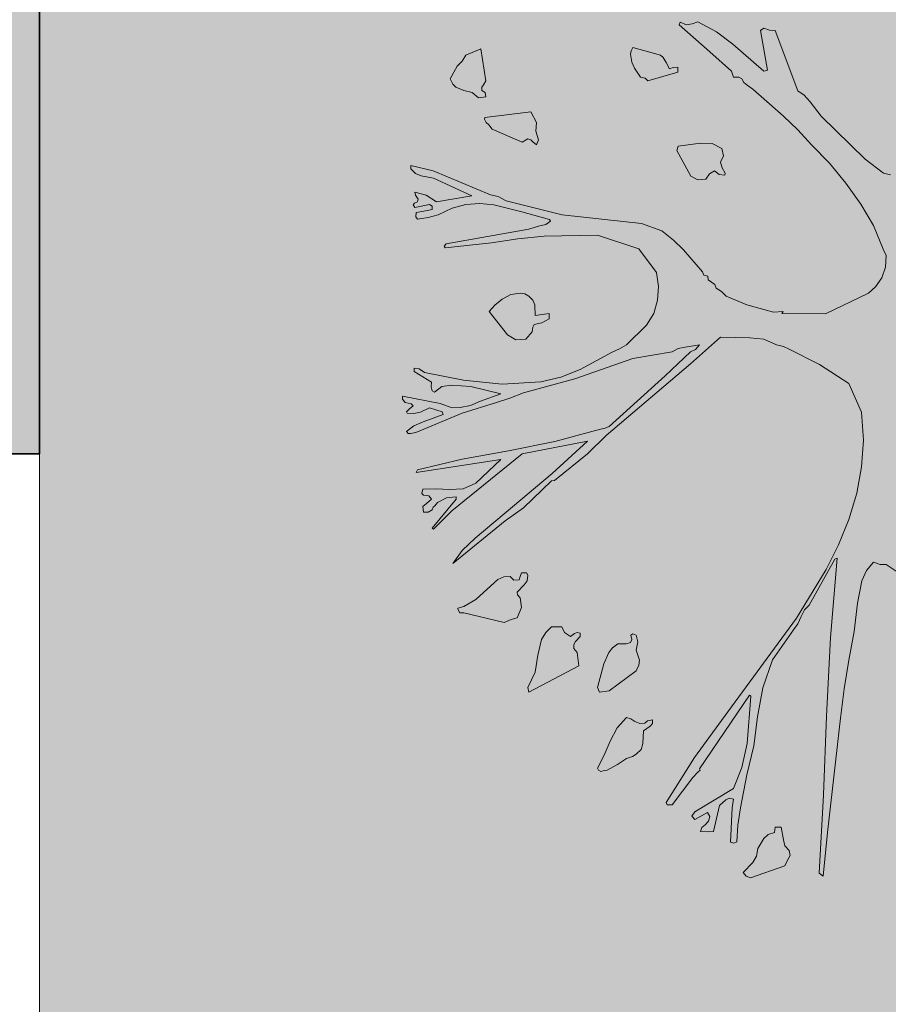
# Model space of a CAD drawing. Units: inches. Extents: x 84 to 1044, y -280 to 906.
# Tile 75 of 105: x 704 to 720, y 481 to 500. Entities that reach past the tile are written whole.
import ezdxf

# ---------------------------------------------------------------- set-up
doc = ezdxf.new("R2010")
doc.units = ezdxf.units.IN
for name, color, linetype, lineweight in [('A-ANNO-DIMS', 2, 'Continuous', 18), ('L-PLNT', 114, 'Continuous', 15), ('WALL', 250, 'Continuous', 35), ('WINDOW', 160, 'Continuous', 13)]:
    doc.layers.add(name, color=color, linetype=linetype, lineweight=lineweight)
doc.layers.add('A-WALL-PATT', color=251, linetype='Continuous', lineweight=9, true_color=0x636466)
doc.layers.add('L-PLNT-PATT', color=9, linetype='Continuous', lineweight=9, true_color=0xafd9aa)
doc.styles.get("Standard").update_dxf_attribs({"font": 'arial.ttf'})
doc.dimstyles.get("Standard").update_dxf_attribs({"dimtxt": 0.18, "dimasz": 0.18, "dimexe": 0.18, "dimexo": 0.0625, "dimgap": 0.09, "dimtad": 0, "dimtih": 1, "dimtoh": 1, "dimdec": 4, "dimzin": 0, "dimdsep": 46, "dimtxsty": 'Standard', "dimcen": 0.09, "dimadec": 0, "dimazin": 0, "dimtfac": 1, "dimtdec": 4, "dimtofl": 0, "dimtmove": 0, "dimatfit": 3, "dimfxl": 1, "dimtolj": 1, "dimtzin": 0, "dimarcsym": 0})

# ---------------------------------------------------------------- blocks, each defined once
blk = doc.blocks.new('A$C37E508DF')
for p, q in [((0.3456, 1.093), (0.3469, 1.0964)), ((0.3469, 1.0964), (0.355, 1.093)), ((0.3619, 1.0943), (0.3692, 1.0968)), ((0.3692, 1.0968), (0.3923, 1.0844)), ((0.3842, 1.0591), (0.3456, 1.093)), ((0.355, 1.093), (0.3619, 1.0943)), ((0.3923, 1.0844), (0.4129, 1.069)), ((0.4472, 1.0857), (0.4515, 1.0887)), ((0.4562, 1.0364), (0.4472, 1.0857)), ((0.4515, 1.0887), (0.4584, 1.0865)), ((0.4584, 1.0865), (0.4657, 1.0861)), ((0.4657, 1.0861), (0.4939, 1.0107)), ((0.0789, 1.0552), (0.0978, 1.063)), ((0.0978, 1.063), (0.1042, 1.0231)), ((0.2847, 1.0565), (0.2856, 1.0604)), ((0.2856, 1.0604), (0.2877, 1.0647)), ((0.2877, 1.0647), (0.3224, 1.0552)), ((0.4112, 1.0351), (0.3842, 1.0591)), ((0.4129, 1.069), (0.4515, 1.0351)), ((0.0682, 1.0415), (0.0746, 1.0475)), ((0.0746, 1.0475), (0.0789, 1.0552)), ((0.2851, 1.054), (0.2847, 1.0565)), ((0.2864, 1.0463), (0.2851, 1.054)), ((0.2899, 1.039), (0.2864, 1.0463)), ((0.3224, 1.0552), (0.3255, 1.0522)), ((0.3255, 1.0522), (0.3293, 1.0458)), ((0.3293, 1.0458), (0.3336, 1.0381)), ((0.0596, 1.0257), (0.0682, 1.0415)), ((0.2972, 1.0274), (0.2899, 1.039)), ((0.3439, 1.0338), (0.3066, 1.0231)), ((0.3336, 1.0381), (0.3383, 1.0398)), ((0.3383, 1.0398), (0.3439, 1.0402)), ((0.3439, 1.0402), (0.3439, 1.0338)), ((0.4138, 1.0274), (0.4112, 1.0351)), ((0.4515, 1.0351), (0.4562, 1.0364)), ((0.0626, 1.0188), (0.0596, 1.0257)), ((0.1042, 1.0231), (0.1012, 1.018)), ((0.3032, 1.0265), (0.2972, 1.0274)), ((0.3066, 1.0231), (0.3032, 1.0265)), ((0.4202, 1.0274), (0.4138, 1.0274)), ((0.4241, 1.0257), (0.4202, 1.0274)), ((0.4267, 1.0209), (0.4241, 1.0257)), ((0.0665, 1.0149), (0.0626, 1.0188)), ((0.0763, 1.0111), (0.0665, 1.0149)), ((0.087, 1.0085), (0.0763, 1.0111)), ((0.1012, 1.018), (0.099, 1.0149)), ((0.099, 1.0149), (0.099, 1.0111)), ((0.099, 1.0111), (0.1033, 1.0085)), ((0.4305, 1.0175), (0.4267, 1.0209)), ((0.4378, 1.0124), (0.4305, 1.0175)), ((0.476, 0.9789), (0.4378, 1.0124)), ((0.4939, 1.0107), (0.5021, 1.0051)), ((0.0948, 1.0016), (0.087, 1.0085)), ((0.1042, 1.0029), (0.0948, 1.0016)), ((0.1033, 1.0085), (0.1042, 1.0029)), ((0.5021, 1.0051), (0.5094, 0.9969)), ((0.5094, 0.9969), (0.5231, 0.9789)), ((0.1025, 0.9751), (0.1029, 0.9772)), ((0.1046, 0.9708), (0.1025, 0.9751)), ((0.1029, 0.9772), (0.1604, 0.9841)), ((0.1604, 0.9841), (0.1672, 0.9708)), ((0.4939, 0.9618), (0.476, 0.9789)), ((0.5231, 0.9789), (0.578, 0.9253)), ((0.1076, 0.9682), (0.1046, 0.9708)), ((0.1119, 0.9626), (0.1076, 0.9682)), ((0.1496, 0.9463), (0.1119, 0.9626)), ((0.1672, 0.9708), (0.1664, 0.9601)), ((0.1664, 0.9601), (0.1698, 0.9493)), ((0.5111, 0.9429), (0.4939, 0.9618)), ((0.1565, 0.9506), (0.1496, 0.9463)), ((0.1604, 0.9493), (0.1565, 0.9506)), ((0.1629, 0.9468), (0.1604, 0.9493)), ((0.1698, 0.9493), (0.1672, 0.9429)), ((0.1672, 0.9429), (0.1629, 0.9468)), ((0.3426, 0.936), (0.3443, 0.9412)), ((0.3602, 0.9039), (0.3426, 0.936)), ((0.3443, 0.9412), (0.3722, 0.9451)), ((0.3722, 0.9451), (0.3868, 0.9446)), ((0.3868, 0.9446), (0.3992, 0.9386)), ((0.3992, 0.9386), (0.4009, 0.9292)), ((0.5334, 0.9202), (0.5111, 0.9429)), ((0.4009, 0.9292), (0.3975, 0.9215)), ((0.578, 0.9253), (0.6011, 0.9077)), ((0.0103, 0.9129), (0.0103, 0.9172)), ((0.0103, 0.9172), (0.0382, 0.9107)), ((0.0159, 0.9073), (0.0103, 0.9129)), ((0.0382, 0.9107), (0.1098, 0.8807)), ((0.3898, 0.9107), (0.3838, 0.9069)), ((0.3958, 0.906), (0.3898, 0.9107)), ((0.3975, 0.9215), (0.3996, 0.9142)), ((0.3996, 0.9142), (0.4031, 0.9077)), ((0.554, 0.8953), (0.5334, 0.9202)), ((0.0232, 0.9043), (0.0159, 0.9073)), ((0.0386, 0.9013), (0.0232, 0.9043)), ((0.0866, 0.8794), (0.0386, 0.9013)), ((0.3692, 0.8992), (0.3602, 0.9039)), ((0.379, 0.9), (0.3692, 0.8992)), ((0.3838, 0.9069), (0.379, 0.9)), ((0.4026, 0.9052), (0.3958, 0.906)), ((0.4031, 0.9077), (0.4026, 0.9052)), ((0.6011, 0.9077), (0.6097, 0.9056)), ((0.5728, 0.8691), (0.554, 0.8953)), ((0.0159, 0.8803), (0.0154, 0.8837)), ((0.0154, 0.8837), (0.0292, 0.8803)), ((0.0176, 0.8777), (0.0159, 0.8803)), ((0.0193, 0.8752), (0.0176, 0.8777)), ((0.0184, 0.8717), (0.0193, 0.8752)), ((0.0292, 0.8803), (0.0424, 0.8717)), ((0.0424, 0.8717), (0.0866, 0.8794)), ((0.1098, 0.8807), (0.1196, 0.8786)), ((0.1196, 0.8786), (0.1295, 0.873)), ((0.0133, 0.8679), (0.015, 0.87)), ((0.0154, 0.8649), (0.0133, 0.8679)), ((0.015, 0.87), (0.0184, 0.8717)), ((0.0334, 0.8687), (0.0154, 0.8649)), ((0.0266, 0.8602), (0.0369, 0.8623)), ((0.0369, 0.8666), (0.0334, 0.8687)), ((0.0369, 0.8623), (0.0369, 0.8666)), ((0.0617, 0.864), (0.0442, 0.8554)), ((0.0789, 0.8687), (0.0617, 0.864)), ((0.0965, 0.8696), (0.0789, 0.8687)), ((0.1141, 0.8679), (0.0965, 0.8696)), ((0.1492, 0.8593), (0.1141, 0.8679)), ((0.1295, 0.873), (0.1994, 0.8554)), ((0.5887, 0.8421), (0.5728, 0.8691)), ((0.0163, 0.8529), (0.0171, 0.8584)), ((0.0184, 0.8503), (0.0163, 0.8529)), ((0.0171, 0.8584), (0.0266, 0.8602)), ((0.0317, 0.8524), (0.0184, 0.8503)), ((0.0442, 0.8554), (0.0317, 0.8524)), ((0.1835, 0.8499), (0.1492, 0.8593)), ((0.1848, 0.8477), (0.1835, 0.8499)), ((0.1994, 0.8554), (0.2984, 0.8447)), ((0.0545, 0.8194), (0.1578, 0.8378)), ((0.1578, 0.8378), (0.1698, 0.8413)), ((0.1698, 0.8413), (0.1792, 0.8434)), ((0.1792, 0.8434), (0.1848, 0.8477)), ((0.2984, 0.8447), (0.3242, 0.8357)), ((0.6007, 0.8125), (0.5887, 0.8421)), ((0.1441, 0.8258), (0.1111, 0.8207)), ((0.1771, 0.8288), (0.1441, 0.8258)), ((0.2436, 0.8301), (0.1771, 0.8288)), ((0.2954, 0.813), (0.2436, 0.8301)), ((0.3242, 0.8357), (0.3387, 0.8241)), ((0.0519, 0.8164), (0.0545, 0.8194)), ((0.0532, 0.8143), (0.0519, 0.8164)), ((0.1111, 0.8207), (0.0532, 0.8143)), ((0.3173, 0.7834), (0.2954, 0.813)), ((0.3387, 0.8241), (0.3512, 0.8117)), ((0.6046, 0.8048), (0.6007, 0.8125)), ((0.3512, 0.8117), (0.3748, 0.7842)), ((0.6037, 0.7903), (0.6046, 0.8048)), ((0.599, 0.777), (0.6037, 0.7903)), ((0.3199, 0.7662), (0.3173, 0.7834)), ((0.3748, 0.7842), (0.3765, 0.7804)), ((0.3765, 0.7804), (0.3816, 0.7791)), ((0.3816, 0.7791), (0.382, 0.7744)), ((0.5913, 0.7658), (0.599, 0.777)), ((0.3186, 0.7491), (0.3199, 0.7662)), ((0.382, 0.7744), (0.3859, 0.7714)), ((0.3859, 0.7714), (0.3902, 0.7684)), ((0.3902, 0.7684), (0.3919, 0.7641)), ((0.3919, 0.7641), (0.3988, 0.7598)), ((0.5823, 0.7577), (0.5913, 0.7658)), ((0.1244, 0.7504), (0.1351, 0.7559)), ((0.1351, 0.7559), (0.1471, 0.7577)), ((0.1471, 0.7577), (0.1527, 0.7568)), ((0.1527, 0.7568), (0.1578, 0.7538)), ((0.1578, 0.7538), (0.1629, 0.7491)), ((0.3988, 0.7598), (0.4043, 0.7538)), ((0.4043, 0.7538), (0.4301, 0.7431)), ((0.5287, 0.7319), (0.5823, 0.7577)), ((0.1081, 0.7349), (0.1153, 0.7427)), ((0.1153, 0.7427), (0.1244, 0.7504)), ((0.1629, 0.7491), (0.1651, 0.7431)), ((0.1651, 0.7431), (0.1655, 0.7298)), ((0.3139, 0.7324), (0.3186, 0.7491)), ((0.4301, 0.7431), (0.4515, 0.7371)), ((0.1312, 0.7058), (0.1081, 0.7349)), ((0.1655, 0.7298), (0.1831, 0.7324)), ((0.1831, 0.7324), (0.1831, 0.7255)), ((0.3049, 0.7178), (0.3139, 0.7324)), ((0.4515, 0.7371), (0.4635, 0.7341)), ((0.4635, 0.7341), (0.4755, 0.7349)), ((0.4755, 0.7349), (0.4742, 0.7324)), ((0.4742, 0.7324), (0.5287, 0.7319)), ((0.1629, 0.7152), (0.1621, 0.7092)), ((0.1646, 0.7186), (0.1629, 0.7152)), ((0.1741, 0.7208), (0.1646, 0.7186)), ((0.1831, 0.7255), (0.1741, 0.7208)), ((0.28, 0.6933), (0.3049, 0.7178)), ((0.1415, 0.6994), (0.1312, 0.7058)), ((0.1621, 0.7092), (0.1539, 0.7002)), ((0.3975, 0.7028), (0.3598, 0.6693)), ((0.4339, 0.7019), (0.3975, 0.7028)), ((0.4515, 0.7002), (0.4339, 0.7019)), ((0.1539, 0.7002), (0.1415, 0.6994)), ((0.271, 0.6882), (0.28, 0.6933)), ((0.3533, 0.6903), (0.3443, 0.6886)), ((0.3709, 0.6933), (0.3533, 0.6903)), ((0.3662, 0.6873), (0.3709, 0.6933)), ((0.4674, 0.6933), (0.4515, 0.7002)), ((0.476, 0.6912), (0.4674, 0.6933)), ((0.4832, 0.6878), (0.476, 0.6912)), ((0.2221, 0.6625), (0.262, 0.6839)), ((0.262, 0.6839), (0.271, 0.6882)), ((0.337, 0.6843), (0.2877, 0.6762)), ((0.328, 0.6543), (0.3598, 0.6843)), ((0.3443, 0.6886), (0.337, 0.6843)), ((0.3598, 0.6843), (0.3662, 0.6873)), ((0.521, 0.6685), (0.4832, 0.6878)), ((0.2877, 0.6762), (0.2152, 0.6505)), ((0.3598, 0.6693), (0.2543, 0.5797)), ((0.5578, 0.6449), (0.521, 0.6685)), ((0.0146, 0.6599), (0.0146, 0.6642)), ((0.0146, 0.6642), (0.0206, 0.6633)), ((0.036, 0.6466), (0.0146, 0.6599)), ((0.0206, 0.6633), (0.0274, 0.6586)), ((0.0274, 0.6586), (0.0759, 0.6492)), ((0.1728, 0.647), (0.1977, 0.6526)), ((0.1977, 0.6526), (0.2221, 0.6625)), ((0.2581, 0.5913), (0.328, 0.6543)), ((0.0356, 0.6406), (0.036, 0.6466)), ((0.0369, 0.6355), (0.0356, 0.6406)), ((0.0489, 0.641), (0.0399, 0.6342)), ((0.0609, 0.6428), (0.0489, 0.641)), ((0.0853, 0.641), (0.0609, 0.6428)), ((0.0759, 0.6492), (0.1244, 0.644)), ((0.1226, 0.632), (0.0853, 0.641)), ((0.1244, 0.644), (0.1728, 0.647)), ((0.2152, 0.6505), (0.1509, 0.6333)), ((0.5737, 0.6089), (0.5578, 0.6449)), ((0, 0.629), (0.0467, 0.62)), ((0, 0.6252), (0, 0.629)), ((0.0399, 0.6342), (0.0369, 0.6355)), ((0.0973, 0.6226), (0.1226, 0.632)), ((0.1509, 0.6333), (0.1342, 0.6265)), ((0.003, 0.6213), (0, 0.6252)), ((0.0069, 0.6204), (0.003, 0.6213)), ((0.0107, 0.6196), (0.0069, 0.6204)), ((0.0086, 0.6132), (0.0133, 0.617)), ((0.0133, 0.617), (0.0107, 0.6196)), ((0.0467, 0.62), (0.0592, 0.6153)), ((0.0592, 0.6153), (0.072, 0.6149)), ((0.072, 0.6149), (0.0849, 0.6175)), ((0.1175, 0.6213), (0.0746, 0.6076)), ((0.0849, 0.6175), (0.0973, 0.6226)), ((0.1342, 0.6265), (0.1175, 0.6213)), ((0.0047, 0.6093), (0.0086, 0.6132)), ((0.0056, 0.6076), (0.0047, 0.6093)), ((0.0141, 0.6072), (0.0056, 0.6076)), ((0.0223, 0.6089), (0.0141, 0.6072)), ((0.0746, 0.6076), (0.0163, 0.5836)), ((0.0334, 0.6145), (0.0223, 0.6089)), ((0.0257, 0.5969), (0.0506, 0.6063)), ((0.0416, 0.6119), (0.0334, 0.6145)), ((0.0493, 0.6093), (0.0416, 0.6119)), ((0.0506, 0.6063), (0.0493, 0.6093)), ((0.5763, 0.5741), (0.5737, 0.6089)), ((0.0047, 0.5849), (0.0141, 0.5921)), ((0.0141, 0.5921), (0.0257, 0.5969)), ((0.253, 0.5892), (0.2581, 0.5913)), ((0.0069, 0.5823), (0.0047, 0.5849)), ((0.0099, 0.5823), (0.0069, 0.5823)), ((0.0163, 0.5836), (0.0099, 0.5823)), ((0.1904, 0.5724), (0.2474, 0.5879)), ((0.2543, 0.5797), (0.2311, 0.557)), ((0.2474, 0.5879), (0.253, 0.5892)), ((0.1325, 0.5608), (0.1904, 0.5724)), ((0.2311, 0.5729), (0.1496, 0.557)), ((0.1869, 0.5325), (0.2311, 0.5729)), ((0.5737, 0.5407), (0.5763, 0.5741)), ((0.1496, 0.557), (0.0613, 0.4858)), ((0.0746, 0.5501), (0.1325, 0.5608)), ((0.2311, 0.557), (0.1899, 0.5235)), ((0.1226, 0.5497), (0.0171, 0.5338)), ((0.0184, 0.5368), (0.0746, 0.5501)), ((0.0917, 0.5205), (0.1226, 0.5497)), ((0.0171, 0.5338), (0.0184, 0.5368)), ((0.1269, 0.482), (0.1869, 0.5325)), ((0.5677, 0.5077), (0.5737, 0.5407)), ((0.0755, 0.5133), (0.0917, 0.5205)), ((0.1861, 0.5231), (0.1509, 0.4897)), ((0.1899, 0.5235), (0.1861, 0.5231)), ((0.024, 0.5072), (0.0253, 0.5128)), ((0.0262, 0.5055), (0.024, 0.5072)), ((0.0253, 0.5128), (0.042, 0.5133)), ((0.0326, 0.5047), (0.0262, 0.5055)), ((0.036, 0.5004), (0.0326, 0.5047)), ((0.042, 0.5133), (0.0587, 0.5124)), ((0.0587, 0.5124), (0.0755, 0.5133)), ((0.5578, 0.4751), (0.5677, 0.5077)), ((0.0253, 0.491), (0.03, 0.4948)), ((0.03, 0.4948), (0.036, 0.5004)), ((0.0369, 0.4639), (0.0669, 0.5004)), ((0.0403, 0.4922), (0.0382, 0.4905)), ((0.0437, 0.4961), (0.0403, 0.4922)), ((0.0549, 0.5021), (0.0437, 0.4961)), ((0.0669, 0.5034), (0.0549, 0.5021)), ((0.0669, 0.5004), (0.0669, 0.5034)), ((0.0262, 0.4841), (0.0253, 0.491)), ((0.0317, 0.4841), (0.0262, 0.4841)), ((0.0369, 0.4871), (0.0317, 0.4841)), ((0.0382, 0.4905), (0.0369, 0.4871)), ((0.0613, 0.4858), (0.0386, 0.4627)), ((0.0905, 0.4515), (0.1269, 0.482)), ((0.1509, 0.4897), (0.1282, 0.4734)), ((0.1282, 0.4734), (0.0626, 0.4198)), ((0.545, 0.4434), (0.5578, 0.4751)), ((0.0386, 0.4627), (0.0369, 0.4639)), ((0.0746, 0.4361), (0.0905, 0.4515)), ((0.5295, 0.4125), (0.545, 0.4434)), ((0.0626, 0.4198), (0.0746, 0.4361)), ((0.5403, 0.4254), (0.5081, 0.3679)), ((0.5347, 0.3276), (0.5433, 0.4266)), ((0.5433, 0.4266), (0.5403, 0.4254)), ((0.5887, 0.4215), (0.5797, 0.4112)), ((0.5969, 0.4189), (0.5887, 0.4215)), ((0.6046, 0.4189), (0.5969, 0.4189)), ((0.6295, 0.4022), (0.6046, 0.4189)), ((0.1471, 0.4035), (0.1484, 0.4082)), ((0.1484, 0.4082), (0.1548, 0.4082)), ((0.1548, 0.4082), (0.1565, 0.4052)), ((0.4922, 0.3516), (0.5295, 0.4125)), ((0.5797, 0.4112), (0.5741, 0.3983)), ((0.1055, 0.388), (0.1192, 0.4001)), ((0.1192, 0.4001), (0.1265, 0.4031)), ((0.1265, 0.4031), (0.1346, 0.4039)), ((0.1346, 0.4039), (0.1389, 0.3992)), ((0.1389, 0.3992), (0.1458, 0.3996)), ((0.1458, 0.3996), (0.1471, 0.4035)), ((0.1556, 0.3983), (0.1518, 0.3932)), ((0.1565, 0.4052), (0.1556, 0.3983)), ((0.5741, 0.3983), (0.5686, 0.3705)), ((0.0917, 0.3748), (0.1055, 0.388)), ((0.1518, 0.3932), (0.1432, 0.3842)), ((0.1432, 0.3842), (0.1436, 0.3808)), ((0.0763, 0.3662), (0.0917, 0.3748)), ((0.1436, 0.3808), (0.1471, 0.3769)), ((0.1471, 0.3769), (0.1484, 0.3649)), ((0.5686, 0.3705), (0.5643, 0.3349)), ((0.069, 0.364), (0.0763, 0.3662)), ((0.069, 0.3627), (0.069, 0.364)), ((0.0716, 0.3585), (0.069, 0.3627)), ((0.0763, 0.3585), (0.0716, 0.3585)), ((0.1269, 0.3464), (0.0763, 0.3585)), ((0.1484, 0.3649), (0.1432, 0.352)), ((0.5025, 0.3619), (0.4982, 0.3537)), ((0.5081, 0.3679), (0.5025, 0.3619)), ((0.1355, 0.3499), (0.1269, 0.3464)), ((0.1432, 0.352), (0.1355, 0.3499)), ((0.4065, 0.2345), (0.4922, 0.3516)), ((0.4939, 0.3447), (0.4884, 0.337)), ((0.4982, 0.3537), (0.4939, 0.3447)), ((0.1737, 0.325), (0.1788, 0.3336)), ((0.1788, 0.3336), (0.1861, 0.3409)), ((0.1861, 0.3409), (0.199, 0.3409)), ((0.199, 0.3409), (0.2024, 0.3336)), ((0.2024, 0.3336), (0.2097, 0.3289)), ((0.2097, 0.3289), (0.2148, 0.3323)), ((0.2148, 0.3323), (0.2182, 0.3336)), ((0.2182, 0.3336), (0.2221, 0.3327)), ((0.2221, 0.3327), (0.2221, 0.3289)), ((0.4884, 0.337), (0.4622, 0.2997)), ((0.5643, 0.3349), (0.5578, 0.2993)), ((0.1689, 0.3053), (0.1737, 0.325)), ((0.2161, 0.3224), (0.214, 0.3186)), ((0.2221, 0.3289), (0.2161, 0.3224)), ((0.2796, 0.3194), (0.2847, 0.3211)), ((0.2847, 0.3211), (0.2864, 0.325)), ((0.2851, 0.3302), (0.2877, 0.3319)), ((0.2864, 0.325), (0.2851, 0.3302)), ((0.2877, 0.3319), (0.292, 0.3306)), ((0.292, 0.3306), (0.2941, 0.322)), ((0.2941, 0.322), (0.292, 0.3117)), ((0.53, 0.229), (0.5347, 0.3276)), ((0.214, 0.3186), (0.214, 0.3139)), ((0.214, 0.3139), (0.2182, 0.3087)), ((0.2182, 0.3087), (0.2204, 0.292)), ((0.2517, 0.2946), (0.2577, 0.3087)), ((0.2577, 0.3087), (0.2624, 0.3147)), ((0.2624, 0.3147), (0.2689, 0.3194)), ((0.2689, 0.3194), (0.2796, 0.3194)), ((0.292, 0.3117), (0.2959, 0.2993)), ((0.1655, 0.2843), (0.1689, 0.3053)), ((0.2959, 0.2993), (0.2954, 0.2928)), ((0.4622, 0.2997), (0.4502, 0.2645)), ((0.5578, 0.2993), (0.5518, 0.2633)), ((0.1565, 0.265), (0.1655, 0.2843)), ((0.2204, 0.292), (0.1578, 0.259)), ((0.2436, 0.265), (0.2517, 0.2946)), ((0.292, 0.286), (0.2581, 0.2607)), ((0.2954, 0.2928), (0.292, 0.286)), ((0.1578, 0.259), (0.1565, 0.265)), ((0.2461, 0.259), (0.2436, 0.265)), ((0.2581, 0.2607), (0.2461, 0.259)), ((0.4502, 0.2645), (0.4438, 0.2285)), ((0.5518, 0.2633), (0.5475, 0.2268)), ((0.4335, 0.2556), (0.3709, 0.1634)), ((0.4305, 0.1951), (0.4352, 0.2543)), ((0.4352, 0.2543), (0.4335, 0.2556)), ((0.3649, 0.1775), (0.4065, 0.2345)), ((0.268, 0.2148), (0.28, 0.2277)), ((0.28, 0.2277), (0.2851, 0.226)), ((0.2851, 0.226), (0.2903, 0.2225)), ((0.2903, 0.2225), (0.2963, 0.22)), ((0.3027, 0.2204), (0.3061, 0.2234)), ((0.3061, 0.2234), (0.3122, 0.2247)), ((0.3122, 0.2247), (0.3122, 0.22)), ((0.4438, 0.2285), (0.4391, 0.1921)), ((0.5261, 0.1308), (0.53, 0.229)), ((0.5475, 0.2268), (0.5313, 0.084)), ((0.2594, 0.1981), (0.268, 0.2148)), ((0.2963, 0.22), (0.3027, 0.2204)), ((0.301, 0.211), (0.3002, 0.1951)), ((0.3096, 0.2165), (0.301, 0.211)), ((0.3122, 0.22), (0.3096, 0.2165)), ((0.2521, 0.1805), (0.2594, 0.1981)), ((0.298, 0.1874), (0.292, 0.1818)), ((0.3002, 0.1951), (0.298, 0.1874)), ((0.4241, 0.1651), (0.4305, 0.1951)), ((0.4391, 0.1921), (0.4301, 0.1561)), ((0.2436, 0.1642), (0.2521, 0.1805)), ((0.28, 0.1762), (0.2684, 0.1689)), ((0.2873, 0.1788), (0.28, 0.1762)), ((0.292, 0.1818), (0.2873, 0.1788)), ((0.3293, 0.1213), (0.3649, 0.1775)), ((0.2448, 0.1616), (0.2436, 0.1642)), ((0.2478, 0.1599), (0.2448, 0.1616)), ((0.2508, 0.1608), (0.2478, 0.1599)), ((0.2556, 0.1616), (0.2508, 0.1608)), ((0.2684, 0.1689), (0.2556, 0.1616)), ((0.3718, 0.1616), (0.3692, 0.1591)), ((0.3709, 0.1634), (0.3718, 0.1616)), ((0.4138, 0.1389), (0.4241, 0.1651)), ((0.3628, 0.1526), (0.337, 0.1183)), ((0.3692, 0.1591), (0.3628, 0.1526)), ((0.4301, 0.1561), (0.4224, 0.1145)), ((0.3653, 0.1098), (0.4138, 0.1389)), ((0.4039, 0.1248), (0.3962, 0.1175)), ((0.4082, 0.1269), (0.4039, 0.1248)), ((0.4134, 0.1256), (0.4082, 0.1269)), ((0.4121, 0.1145), (0.4134, 0.1256)), ((0.5205, 0.033), (0.5261, 0.1308)), ((0.3306, 0.1183), (0.3293, 0.1213)), ((0.337, 0.1183), (0.3306, 0.1183)), ((0.3962, 0.1175), (0.3885, 0.0853)), ((0.4099, 0.0716), (0.4121, 0.1145)), ((0.4224, 0.1145), (0.4189, 0.093)), ((0.3615, 0.1042), (0.3653, 0.1098)), ((0.3653, 0.0999), (0.3615, 0.1042)), ((0.3812, 0.1089), (0.3653, 0.0999)), ((0.3842, 0.1037), (0.3812, 0.1089)), ((0.3825, 0.0978), (0.3842, 0.1037)), ((0.3722, 0.0853), (0.3739, 0.09)), ((0.3739, 0.09), (0.3782, 0.0935)), ((0.3782, 0.0935), (0.3825, 0.0978)), ((0.4189, 0.093), (0.4176, 0.072)), ((0.4648, 0.084), (0.4657, 0.0905)), ((0.4657, 0.0905), (0.473, 0.0905)), ((0.473, 0.0905), (0.476, 0.0746)), ((0.3808, 0.0845), (0.3722, 0.0853)), ((0.3885, 0.0853), (0.3808, 0.0845)), ((0.4442, 0.0639), (0.4515, 0.0763)), ((0.4515, 0.0763), (0.4571, 0.0815)), ((0.4571, 0.0815), (0.4648, 0.084)), ((0.476, 0.0746), (0.4777, 0.0673)), ((0.5313, 0.084), (0.5257, 0.0291)), ((0.4142, 0.0707), (0.4099, 0.0716)), ((0.4176, 0.072), (0.4142, 0.0707)), ((0.4425, 0.0544), (0.4442, 0.0639)), ((0.4777, 0.0673), (0.4832, 0.0613)), ((0.4378, 0.0463), (0.4425, 0.0544)), ((0.4811, 0.0493), (0.4777, 0.0424)), ((0.4845, 0.0553), (0.4811, 0.0493)), ((0.4832, 0.0613), (0.4845, 0.0553)), ((0.4258, 0.0339), (0.4378, 0.0463)), ((0.4777, 0.0424), (0.4348, 0.0274)), ((0.4296, 0.0291), (0.4258, 0.0339)), ((0.4348, 0.0274), (0.4296, 0.0291)), ((0.5257, 0.0291), (0.5205, 0.033))]:
    blk.add_line(p, q)
blk = doc.blocks.new('WIN-72IN')
blk.add_line((72.004, 9), (0.004, 9))
blk = doc.blocks.new('*D62')
at = {"layer": 'A-ANNO-DIMS', "color": 0, "lineweight": -2, "transparency": 16777216}
for p, q in [((203.179, 709.183), (203.179, 905.9)), ((896.074, 400.183), (896.074, 905.9)), ((203.359, 905.72), (549.232, 905.72)), ((895.894, 905.72), (550.021, 905.72))]:
    blk.add_line(p, q, dxfattribs=at)
at = {"layer": 'A-ANNO-DIMS', "color": 0, "transparency": 16777216}
for points in [[(203.359, 905.75), (203.359, 905.69), (203.179, 905.72)], [(895.894, 905.75), (895.894, 905.69), (896.074, 905.72)]]:
    blk.add_solid(points, dxfattribs=at)
at = {"layer": 'Defpoints', "color": 0, "transparency": 16777216}
for p in [(896.074, 905.72), (203.179, 709.12), (896.074, 400.12)]:
    blk.add_point(p, dxfattribs=at)
at = {"layer": 'A-ANNO-DIMS', "color": 0, "transparency": 16777216, "insert": (549.627, 905.72), "char_height": 0.18, "attachment_point": 5}
blk.add_mtext('\\A1;692.9', dxfattribs=at)

msp = doc.modelspace()

# ---------------------------------------------------------------- hatches: boundary and pattern name
at = {"layer": 'A-WALL-PATT', "transparency": 33554597}
h = msp.add_hatch(color=256, dxfattribs=at)
h.dxf.hatch_style = 1
h.paths.add_polyline_path([(671.074, 100.12), (647.074, 100.12), (647.074, 160.12), (641.074, 160.12), (620.824, 160.12), (620.824, 151.12), (638.074, 151.12), (638.074, 91.12), (671.074, 91.12)])
h.paths.add_polyline_path([(791.074, 100.12), (743.074, 100.12), (743.074, 91.12), (791.074, 91.12)])
h.paths.add_polyline_path([(896.074, 346.12), (887.074, 346.12), (887.074, 334.12), (870.955, 334.12), (833.074, 334.12), (804.574, 334.12), (804.574, 328.12), (887.074, 328.12), (887.074, 100.12), (863.074, 100.12), (863.074, 91.12), (896.074, 91.12)])
h.paths.add_polyline_path([(507.574, 154.729), (507.574, 160.12), (464.074, 160.12), (464.074, 247.12), (641.074, 247.12), (641.074, 208.12), (647.074, 208.12), (647.074, 328.12), (659.074, 328.12), (659.074, 334.12), (617.074, 334.12), (617.074, 328.12), (641.074, 328.12), (641.074, 256.12), (545.074, 256.12), (545.074, 328.12), (569.074, 328.12), (569.074, 334.12), (518.074, 334.12), (518.074, 325.12), (536.074, 325.12), (536.074, 256.12), (464.074, 256.12), (464.074, 325.12), (482.074, 325.12), (482.074, 334.12), (455.074, 334.12), (455.074, 160.12), (413.127, 160.12), (413.127, 151.12), (455.074, 151.12), (455.074, 91.12), (464.074, 91.12), (464.074, 151.12), (507.574, 151.12)])
h.paths.add_polyline_path([(572.824, 160.12), (555.574, 160.12), (555.574, 151.12), (572.824, 151.12)], flags=17)
h.paths.add_polyline_path([(341.127, 160.12), (299.179, 160.12), (299.179, 211.12), (294.179, 211.12), (290.179, 211.12), (290.179, 151.12), (341.127, 151.12)])
h.paths.add_polyline_path([(299.179, 256.12), (212.179, 256.12), (212.179, 274.12), (203.179, 274.12), (203.179, 247.12), (299.179, 247.12)])
h.paths.add_polyline_path([(212.179, 514.12), (398.074, 514.12), (398.074, 519.12), (398.074, 520.12), (212.179, 520.12), (212.179, 574.12), (203.179, 574.12), (203.179, 310.12), (212.179, 310.12), (212.179, 328.12), (290.179, 328.12), (290.179, 292.12), (299.179, 292.12), (299.179, 328.12), (332.179, 328.12), (332.179, 334.12), (212.179, 334.12)])
h.paths.add_polyline_path([(287.127, 709.12), (203.179, 709.12), (203.179, 646.12), (212.179, 646.12), (212.179, 700.12), (287.127, 700.12)])
h.paths.add_polyline_path([(470.074, 709.12), (359.127, 709.12), (359.127, 700.12), (434.074, 700.12), (434.074, 574.12), (440.074, 574.12), (440.074, 622.12), (464.074, 622.12), (464.074, 628.12), (440.074, 628.12), (440.074, 700.12), (470.074, 700.12)])
h.paths.add_polyline_path([(572.074, 709.12), (506.074, 709.12), (506.074, 700.12), (536.074, 700.12), (536.074, 628.12), (494.074, 628.12), (494.074, 622.12), (536.074, 622.12), (536.074, 520.12), (440.074, 520.12), (440.074, 544.12), (434.074, 544.12), (434.074, 514.12), (644.074, 514.12), (644.074, 519.12), (644.074, 544.12), (638.074, 544.12), (638.074, 520.12), (542.074, 520.12), (542.074, 622.12), (584.074, 622.12), (584.074, 628.12), (542.074, 628.12), (542.074, 700.12), (572.074, 700.12)])
h.paths.add_polyline_path([(698.074, 709.12), (608.074, 709.12), (608.074, 700.12), (638.074, 700.12), (638.074, 628.12), (614.074, 628.12), (614.074, 622.12), (638.074, 622.12), (638.074, 574.12), (644.074, 574.12), (644.074, 700.12), (698.074, 700.12)])
h.paths.add_polyline_path([(833.074, 709.12), (770.074, 709.12), (770.074, 700.12), (824.074, 700.12), (824.074, 646.12), (833.074, 646.12)])
h.paths.add_polyline_path([(833.074, 574.12), (824.074, 574.12), (824.074, 520.12), (791.244, 520.12), (712.904, 520.12), (680.074, 520.12), (680.074, 514.12), (695.074, 514.12), (695.074, 491.62), (704.074, 491.62), (704.074, 511.12), (833.074, 511.12)])
h.paths.add_polyline_path([(704.074, 419.62), (695.074, 419.62), (695.074, 370.12), (704.074, 370.12)])
h.paths.add_polyline_path([(896.074, 400.12), (833.074, 400.12), (833.074, 364.12), (839.074, 364.12), (839.074, 394.12), (887.074, 394.12), (887.074, 382.12), (896.074, 382.12)])
h.paths.add_polyline_path([(732.574, 334.12), (695.074, 334.12), (695.074, 328.12), (732.574, 328.12)])
at = {"layer": 'L-PLNT-PATT', "transparency": 33554597}
h = msp.add_hatch(color=256, dxfattribs=at)
h.dxf.hatch_style = 1
h.paths.add_polyline_path([(896.074, 511.12), (704.074, 511.12), (704.074, 491.62), (704.074, 419.62), (704.074, 400.12), (833.074, 400.12), (896.074, 400.12)])

# ---------------------------------------------------------------- linework, layer by layer
at = {"layer": 'WALL'}
for q in [(704.074, 511.12), (695.074, 491.62)]:
    msp.add_line((704.074, 491.62), q, dxfattribs=at)

# ---------------------------------------------------------------- block references
at = {"layer": 'L-PLNT', "xscale": 15.19586232982809, "yscale": 15.19586232982809, "zscale": 15.19586232982809}
msp.add_blockref('A$C37E508DF', (710.97, 483.159), dxfattribs=at)
at = {"layer": 'WINDOW', "rotation": 270.0000000000001}
msp.add_blockref('WIN-72IN', (695.074, 491.624), dxfattribs=at)

# ---------------------------------------------------------------- dimensions: what is measured, and where the dimension line sits
at = {"layer": 'A-ANNO-DIMS'}
dim = msp.add_linear_dim(base=(896.074, 905.72), p1=(203.179, 709.12), p2=(896.074, 400.12), dimstyle='Standard', override={"dimdec": 1, "dimlfac": 1, "dimrnd": 0, "dimzin": 0, "dimdsep": 46, "dimlunit": 2}, dxfattribs=at)
dim.commit()
dim.dimension.update_dxf_attribs({"geometry": '*D62', "text_midpoint": (549.627, 905.72)})

doc.saveas('drawing.dxf')
